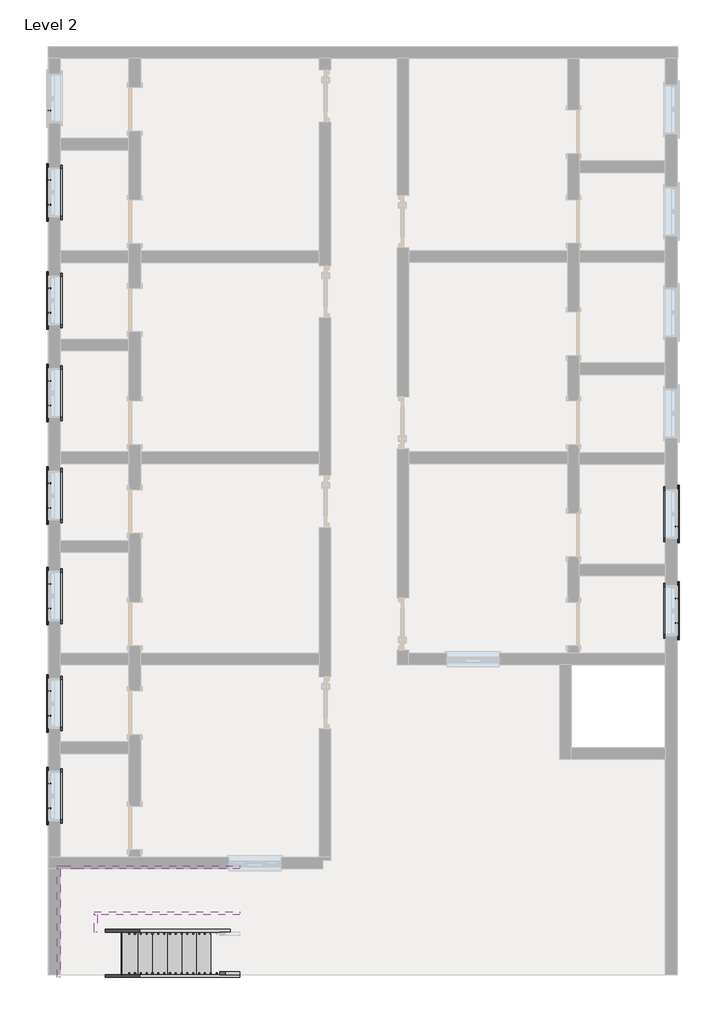
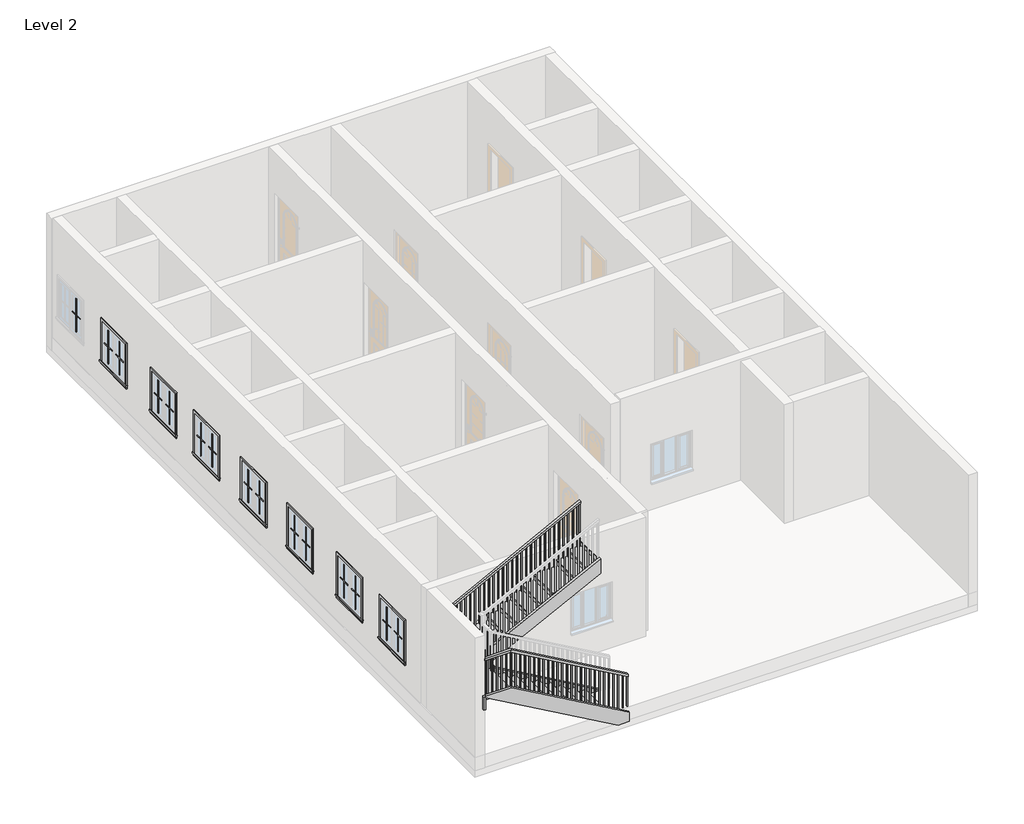
# One storey, part 3 of 4: 36 proxies, 6 members, 1 railing, 1 stair flight.
"""IFC4 building model written with IfcOpenShell, lengths in millimetres."""

from ifc_helpers import new_model, si_unit, frame, origin, place, context, project, spatial, polyline, outline, extrude, faceted_brep, transform, mapped, element, save
from components import muntin_pattern_2x2_muntin_pattern_2x2_b3fe6957, muntin_pattern_2x2_muntin_pattern_2x2_3e0ecaf2, trim_window_exterior_flat_with_sill_41619996, trim_window_interior_flat_picture_frame_51c85655, stair_flight_618316a1

model = new_model("IFC4")

# Units and contexts
model_context = context("Model", 3, world=origin())
ifc_project = project(units=[si_unit("LENGTHUNIT", "METRE", prefix="MILLI")], contexts=[model_context])

# Site, building, storey
site = spatial("IfcSite", under=ifc_project)
building = spatial("IfcBuilding", under=site)
storey = spatial("IfcBuildingStorey", under=building, Name="Level 2", Elevation=3048.0)

# Proxies
placement = place(None, origin())
muntin_pattern_2x2_muntin_pattern_2x2_shape = muntin_pattern_2x2_muntin_pattern_2x2_b3fe6957(model_context)
element("IfcBuildingElementProxy", 1, Name="Muntin Pattern_2x2 : Muntin Pattern_2x2", ObjectType="Muntin Pattern_2x2 : Muntin Pattern_2x2", at=placement, inside=storey, context=model_context, shape_type="MappedRepresentation", body=[
    mapped(muntin_pattern_2x2_muntin_pattern_2x2_shape, transform((-6438.8858866, 6882.8274728, 4032.25), x_axis=(0.0, 1.0, 0.0), y_axis=(-1.0, 0.0, 0.0), z_axis=(0.0, 0.0, 1.0))),
])
element("IfcBuildingElementProxy", 2, Name="Muntin Pattern_2x2 : Muntin Pattern_2x2", ObjectType="Muntin Pattern_2x2 : Muntin Pattern_2x2", at=placement, inside=storey, context=model_context, shape_type="MappedRepresentation", body=[
    mapped(muntin_pattern_2x2_muntin_pattern_2x2_shape, transform((-6438.8858866, 5244.5274728, 4032.25), x_axis=(0.0, 1.0, 0.0), y_axis=(-1.0, 0.0, 0.0), z_axis=(0.0, 0.0, 1.0))),
])
element("IfcBuildingElementProxy", 3, Name="Muntin Pattern_2x2 : Muntin Pattern_2x2", ObjectType="Muntin Pattern_2x2 : Muntin Pattern_2x2", at=placement, inside=storey, context=model_context, shape_type="MappedRepresentation", body=[
    mapped(muntin_pattern_2x2_muntin_pattern_2x2_shape, transform((-6438.8858866, 3360.4810874, 4032.25), x_axis=(0.0, 1.0, 0.0), y_axis=(-1.0, 0.0, 0.0), z_axis=(0.0, 0.0, 1.0))),
])
element("IfcBuildingElementProxy", 4, Name="Muntin Pattern_2x2 : Muntin Pattern_2x2", ObjectType="Muntin Pattern_2x2 : Muntin Pattern_2x2", at=placement, inside=storey, context=model_context, shape_type="MappedRepresentation", body=[
    mapped(muntin_pattern_2x2_muntin_pattern_2x2_shape, transform((-6438.8858866, 1745.426343, 4032.25), x_axis=(0.0, 1.0, 0.0), y_axis=(-1.0, 0.0, 0.0), z_axis=(0.0, 0.0, 1.0))),
])
element("IfcBuildingElementProxy", 5, Name="Muntin Pattern_2x2 : Muntin Pattern_2x2", ObjectType="Muntin Pattern_2x2 : Muntin Pattern_2x2", at=placement, inside=storey, context=model_context, shape_type="MappedRepresentation", body=[
    mapped(muntin_pattern_2x2_muntin_pattern_2x2_shape, transform((-6438.8858866, -38.6725272, 4032.25), x_axis=(0.0, 1.0, 0.0), y_axis=(-1.0, 0.0, 0.0), z_axis=(0.0, 0.0, 1.0))),
])
element("IfcBuildingElementProxy", 6, Name="Muntin Pattern_2x2 : Muntin Pattern_2x2", ObjectType="Muntin Pattern_2x2 : Muntin Pattern_2x2", at=placement, inside=storey, context=model_context, shape_type="MappedRepresentation", body=[
    mapped(muntin_pattern_2x2_muntin_pattern_2x2_shape, transform((-6438.8858866, -1791.2725272, 4032.25), x_axis=(0.0, 1.0, 0.0), y_axis=(-1.0, 0.0, 0.0), z_axis=(0.0, 0.0, 1.0))),
])
element("IfcBuildingElementProxy", 7, Name="Muntin Pattern_2x2 : Muntin Pattern_2x2", ObjectType="Muntin Pattern_2x2 : Muntin Pattern_2x2", at=placement, inside=storey, context=model_context, shape_type="MappedRepresentation", body=[
    mapped(muntin_pattern_2x2_muntin_pattern_2x2_shape, transform((-6438.8858866, -3658.1725272, 4032.25), x_axis=(0.0, 1.0, 0.0), y_axis=(-1.0, 0.0, 0.0), z_axis=(0.0, 0.0, 1.0))),
])
element("IfcBuildingElementProxy", 8, Name="Muntin Pattern_2x2 : Muntin Pattern_2x2", ObjectType="Muntin Pattern_2x2 : Muntin Pattern_2x2", at=placement, inside=storey, context=model_context, shape_type="MappedRepresentation", body=[
    mapped(muntin_pattern_2x2_muntin_pattern_2x2_shape, transform((-6438.8858866, -5271.0725272, 4032.25), x_axis=(0.0, 1.0, 0.0), y_axis=(-1.0, 0.0, 0.0), z_axis=(0.0, 0.0, 1.0))),
])
element("IfcBuildingElementProxy", 9, Name="Muntin Pattern_2x2 : Muntin Pattern_2x2", ObjectType="Muntin Pattern_2x2 : Muntin Pattern_2x2", at=placement, inside=storey, context=model_context, shape_type="MappedRepresentation", body=[
    mapped(muntin_pattern_2x2_muntin_pattern_2x2_shape, transform((4489.4641134, -1616.6475272, 4032.25), x_axis=(0.0, -1.0, 0.0), y_axis=(1.0, 0.0, 0.0), z_axis=(0.0, 0.0, 1.0))),
])
muntin_pattern_2x2_muntin_pattern_2x2_2_shape = muntin_pattern_2x2_muntin_pattern_2x2_3e0ecaf2(model_context)
element("IfcBuildingElementProxy", 10, Name="Muntin Pattern_2x2 : Muntin Pattern_2x2", ObjectType="Muntin Pattern_2x2 : Muntin Pattern_2x2", at=placement, inside=storey, context=model_context, shape_type="MappedRepresentation", body=[
    mapped(muntin_pattern_2x2_muntin_pattern_2x2_2_shape, transform((-6438.8858866, 5673.1524728, 4032.25), x_axis=(0.0, -1.0, 0.0), y_axis=(1.0, 0.0, 0.0), z_axis=(0.0, 0.0, 1.0))),
])
element("IfcBuildingElementProxy", 11, Name="Muntin Pattern_2x2 : Muntin Pattern_2x2", ObjectType="Muntin Pattern_2x2 : Muntin Pattern_2x2", at=placement, inside=storey, context=model_context, shape_type="MappedRepresentation", body=[
    mapped(muntin_pattern_2x2_muntin_pattern_2x2_2_shape, transform((-6438.8858866, 3789.1060874, 4032.25), x_axis=(0.0, -1.0, 0.0), y_axis=(1.0, 0.0, 0.0), z_axis=(0.0, 0.0, 1.0))),
])
element("IfcBuildingElementProxy", 12, Name="Muntin Pattern_2x2 : Muntin Pattern_2x2", ObjectType="Muntin Pattern_2x2 : Muntin Pattern_2x2", at=placement, inside=storey, context=model_context, shape_type="MappedRepresentation", body=[
    mapped(muntin_pattern_2x2_muntin_pattern_2x2_2_shape, transform((-6438.8858866, 2174.051343, 4032.25), x_axis=(0.0, -1.0, 0.0), y_axis=(1.0, 0.0, 0.0), z_axis=(0.0, 0.0, 1.0))),
])
element("IfcBuildingElementProxy", 13, Name="Muntin Pattern_2x2 : Muntin Pattern_2x2", ObjectType="Muntin Pattern_2x2 : Muntin Pattern_2x2", at=placement, inside=storey, context=model_context, shape_type="MappedRepresentation", body=[
    mapped(muntin_pattern_2x2_muntin_pattern_2x2_2_shape, transform((-6438.8858866, 389.9524728, 4032.25), x_axis=(0.0, -1.0, 0.0), y_axis=(1.0, 0.0, 0.0), z_axis=(0.0, 0.0, 1.0))),
])
element("IfcBuildingElementProxy", 14, Name="Muntin Pattern_2x2 : Muntin Pattern_2x2", ObjectType="Muntin Pattern_2x2 : Muntin Pattern_2x2", at=placement, inside=storey, context=model_context, shape_type="MappedRepresentation", body=[
    mapped(muntin_pattern_2x2_muntin_pattern_2x2_2_shape, transform((-6438.8858866, -1362.6475272, 4032.25), x_axis=(0.0, -1.0, 0.0), y_axis=(1.0, 0.0, 0.0), z_axis=(0.0, 0.0, 1.0))),
])
element("IfcBuildingElementProxy", 15, Name="Muntin Pattern_2x2 : Muntin Pattern_2x2", ObjectType="Muntin Pattern_2x2 : Muntin Pattern_2x2", at=placement, inside=storey, context=model_context, shape_type="MappedRepresentation", body=[
    mapped(muntin_pattern_2x2_muntin_pattern_2x2_2_shape, transform((-6438.8858866, -3229.5475272, 4032.25), x_axis=(0.0, -1.0, 0.0), y_axis=(1.0, 0.0, 0.0), z_axis=(0.0, 0.0, 1.0))),
])
element("IfcBuildingElementProxy", 16, Name="Muntin Pattern_2x2 : Muntin Pattern_2x2", ObjectType="Muntin Pattern_2x2 : Muntin Pattern_2x2", at=placement, inside=storey, context=model_context, shape_type="MappedRepresentation", body=[
    mapped(muntin_pattern_2x2_muntin_pattern_2x2_2_shape, transform((-6438.8858866, -4842.4475272, 4032.25), x_axis=(0.0, -1.0, 0.0), y_axis=(1.0, 0.0, 0.0), z_axis=(0.0, 0.0, 1.0))),
])
element("IfcBuildingElementProxy", 17, Name="Muntin Pattern_2x2 : Muntin Pattern_2x2", ObjectType="Muntin Pattern_2x2 : Muntin Pattern_2x2", at=placement, inside=storey, context=model_context, shape_type="MappedRepresentation", body=[
    mapped(muntin_pattern_2x2_muntin_pattern_2x2_2_shape, transform((4489.4641134, -2045.2725272, 4032.25), x_axis=(0.0, 1.0, 0.0), y_axis=(-1.0, 0.0, 0.0), z_axis=(0.0, 0.0, 1.0))),
])
element("IfcBuildingElementProxy", 18, Name="Muntin Pattern_2x2 : Muntin Pattern_2x2", ObjectType="Muntin Pattern_2x2 : Muntin Pattern_2x2", at=placement, inside=storey, context=model_context, shape_type="MappedRepresentation", body=[
    mapped(muntin_pattern_2x2_muntin_pattern_2x2_2_shape, transform((4489.4641134, -362.5225272, 4032.25), x_axis=(0.0, 1.0, 0.0), y_axis=(-1.0, 0.0, 0.0), z_axis=(0.0, 0.0, 1.0))),
])
trim_window_exterior_flat_with_sill_shape = trim_window_exterior_flat_with_sill_41619996(model_context)
element("IfcBuildingElementProxy", 19, Name="Trim-Window-Exterior-Flat : with Sill", ObjectType="Trim-Window-Exterior-Flat : with Sill", at=placement, inside=storey, context=model_context, shape_type="MappedRepresentation", body=[
    mapped(trim_window_exterior_flat_with_sill_shape, transform((-6448.4108866, 5458.8399728, 4876.8), x_axis=(0.0, -1.0, 0.0), y_axis=(0.0, 0.0, 1.0), z_axis=(-1.0, 0.0, 0.0))),
])
element("IfcBuildingElementProxy", 20, Name="Trim-Window-Exterior-Flat : with Sill", ObjectType="Trim-Window-Exterior-Flat : with Sill", at=placement, inside=storey, context=model_context, shape_type="MappedRepresentation", body=[
    mapped(trim_window_exterior_flat_with_sill_shape, transform((-6448.4108866, 3574.7935874, 4876.8), x_axis=(0.0, -1.0, 0.0), y_axis=(0.0, 0.0, 1.0), z_axis=(-1.0, 0.0, 0.0))),
])
element("IfcBuildingElementProxy", 21, Name="Trim-Window-Exterior-Flat : with Sill", ObjectType="Trim-Window-Exterior-Flat : with Sill", at=placement, inside=storey, context=model_context, shape_type="MappedRepresentation", body=[
    mapped(trim_window_exterior_flat_with_sill_shape, transform((-6448.4108866, 1959.738843, 4876.8), x_axis=(0.0, -1.0, 0.0), y_axis=(0.0, 0.0, 1.0), z_axis=(-1.0, 0.0, 0.0))),
])
element("IfcBuildingElementProxy", 22, Name="Trim-Window-Exterior-Flat : with Sill", ObjectType="Trim-Window-Exterior-Flat : with Sill", at=placement, inside=storey, context=model_context, shape_type="MappedRepresentation", body=[
    mapped(trim_window_exterior_flat_with_sill_shape, transform((-6448.4108866, 175.6399728, 4876.8), x_axis=(0.0, -1.0, 0.0), y_axis=(0.0, 0.0, 1.0), z_axis=(-1.0, 0.0, 0.0))),
])
element("IfcBuildingElementProxy", 23, Name="Trim-Window-Exterior-Flat : with Sill", ObjectType="Trim-Window-Exterior-Flat : with Sill", at=placement, inside=storey, context=model_context, shape_type="MappedRepresentation", body=[
    mapped(trim_window_exterior_flat_with_sill_shape, transform((-6448.4108866, -1576.9600272, 4876.8), x_axis=(0.0, -1.0, 0.0), y_axis=(0.0, 0.0, 1.0), z_axis=(-1.0, 0.0, 0.0))),
])
element("IfcBuildingElementProxy", 24, Name="Trim-Window-Exterior-Flat : with Sill", ObjectType="Trim-Window-Exterior-Flat : with Sill", at=placement, inside=storey, context=model_context, shape_type="MappedRepresentation", body=[
    mapped(trim_window_exterior_flat_with_sill_shape, transform((-6448.4108866, -3443.8600272, 4876.8), x_axis=(0.0, -1.0, 0.0), y_axis=(0.0, 0.0, 1.0), z_axis=(-1.0, 0.0, 0.0))),
])
element("IfcBuildingElementProxy", 25, Name="Trim-Window-Exterior-Flat : with Sill", ObjectType="Trim-Window-Exterior-Flat : with Sill", at=placement, inside=storey, context=model_context, shape_type="MappedRepresentation", body=[
    mapped(trim_window_exterior_flat_with_sill_shape, transform((-6448.4108866, -5056.7600272, 4876.8), x_axis=(0.0, -1.0, 0.0), y_axis=(0.0, 0.0, 1.0), z_axis=(-1.0, 0.0, 0.0))),
])
element("IfcBuildingElementProxy", 26, Name="Trim-Window-Exterior-Flat : with Sill", ObjectType="Trim-Window-Exterior-Flat : with Sill", at=placement, inside=storey, context=model_context, shape_type="MappedRepresentation", body=[
    mapped(trim_window_exterior_flat_with_sill_shape, transform((4498.9891134, -1830.9600272, 4876.8), x_axis=(0.0, 1.0, 0.0), y_axis=(0.0, 0.0, 1.0), z_axis=(1.0, 0.0, 0.0))),
])
element("IfcBuildingElementProxy", 27, Name="Trim-Window-Exterior-Flat : with Sill", ObjectType="Trim-Window-Exterior-Flat : with Sill", at=placement, inside=storey, context=model_context, shape_type="MappedRepresentation", body=[
    mapped(trim_window_exterior_flat_with_sill_shape, transform((4498.9891134, -148.2100272, 4876.8), x_axis=(0.0, 1.0, 0.0), y_axis=(0.0, 0.0, 1.0), z_axis=(1.0, 0.0, 0.0))),
])
trim_window_interior_flat_picture_frame_shape = trim_window_interior_flat_picture_frame_51c85655(model_context)
element("IfcBuildingElementProxy", 28, Name="Trim-Window-Interior-Flat : Picture Frame", ObjectType="Trim-Window-Interior-Flat : Picture Frame", at=placement, inside=storey, context=model_context, shape_type="MappedRepresentation", body=[
    mapped(trim_window_interior_flat_picture_frame_shape, transform((-6245.2108866, 5458.8399728, 4876.8), x_axis=(0.0, 1.0, 0.0), y_axis=(0.0, 0.0, 1.0), z_axis=(1.0, 0.0, 0.0))),
])
element("IfcBuildingElementProxy", 29, Name="Trim-Window-Interior-Flat : Picture Frame", ObjectType="Trim-Window-Interior-Flat : Picture Frame", at=placement, inside=storey, context=model_context, shape_type="MappedRepresentation", body=[
    mapped(trim_window_interior_flat_picture_frame_shape, transform((-6245.2108866, 3574.7935874, 4876.8), x_axis=(0.0, 1.0, 0.0), y_axis=(0.0, 0.0, 1.0), z_axis=(1.0, 0.0, 0.0))),
])
element("IfcBuildingElementProxy", 30, Name="Trim-Window-Interior-Flat : Picture Frame", ObjectType="Trim-Window-Interior-Flat : Picture Frame", at=placement, inside=storey, context=model_context, shape_type="MappedRepresentation", body=[
    mapped(trim_window_interior_flat_picture_frame_shape, transform((-6245.2108866, 1959.738843, 4876.8), x_axis=(0.0, 1.0, 0.0), y_axis=(0.0, 0.0, 1.0), z_axis=(1.0, 0.0, 0.0))),
])
element("IfcBuildingElementProxy", 31, Name="Trim-Window-Interior-Flat : Picture Frame", ObjectType="Trim-Window-Interior-Flat : Picture Frame", at=placement, inside=storey, context=model_context, shape_type="MappedRepresentation", body=[
    mapped(trim_window_interior_flat_picture_frame_shape, transform((-6245.2108866, 175.6399728, 4876.8), x_axis=(0.0, 1.0, 0.0), y_axis=(0.0, 0.0, 1.0), z_axis=(1.0, 0.0, 0.0))),
])
element("IfcBuildingElementProxy", 32, Name="Trim-Window-Interior-Flat : Picture Frame", ObjectType="Trim-Window-Interior-Flat : Picture Frame", at=placement, inside=storey, context=model_context, shape_type="MappedRepresentation", body=[
    mapped(trim_window_interior_flat_picture_frame_shape, transform((-6245.2108866, -1576.9600272, 4876.8), x_axis=(0.0, 1.0, 0.0), y_axis=(0.0, 0.0, 1.0), z_axis=(1.0, 0.0, 0.0))),
])
element("IfcBuildingElementProxy", 33, Name="Trim-Window-Interior-Flat : Picture Frame", ObjectType="Trim-Window-Interior-Flat : Picture Frame", at=placement, inside=storey, context=model_context, shape_type="MappedRepresentation", body=[
    mapped(trim_window_interior_flat_picture_frame_shape, transform((-6245.2108866, -3443.8600272, 4876.8), x_axis=(0.0, 1.0, 0.0), y_axis=(0.0, 0.0, 1.0), z_axis=(1.0, 0.0, 0.0))),
])
element("IfcBuildingElementProxy", 34, Name="Trim-Window-Interior-Flat : Picture Frame", ObjectType="Trim-Window-Interior-Flat : Picture Frame", at=placement, inside=storey, context=model_context, shape_type="MappedRepresentation", body=[
    mapped(trim_window_interior_flat_picture_frame_shape, transform((-6245.2108866, -5056.7600272, 4876.8), x_axis=(0.0, 1.0, 0.0), y_axis=(0.0, 0.0, 1.0), z_axis=(1.0, 0.0, 0.0))),
])
element("IfcBuildingElementProxy", 35, Name="Trim-Window-Interior-Flat : Picture Frame", ObjectType="Trim-Window-Interior-Flat : Picture Frame", at=placement, inside=storey, context=model_context, shape_type="MappedRepresentation", body=[
    mapped(trim_window_interior_flat_picture_frame_shape, transform((4295.7891134, -1830.9600272, 4876.8), x_axis=(0.0, -1.0, 0.0), y_axis=(0.0, 0.0, 1.0), z_axis=(-1.0, 0.0, 0.0))),
])
element("IfcBuildingElementProxy", 36, Name="Trim-Window-Interior-Flat : Picture Frame", ObjectType="Trim-Window-Interior-Flat : Picture Frame", at=placement, inside=storey, context=model_context, shape_type="MappedRepresentation", body=[
    mapped(trim_window_interior_flat_picture_frame_shape, transform((4295.7891134, -148.2100272, 4876.8), x_axis=(0.0, -1.0, 0.0), y_axis=(0.0, 0.0, 1.0), z_axis=(-1.0, 0.0, 0.0))),
])

# Members
element("IfcMember", 37, ObjectType="Stringer - 2\" Width", at=placement, inside=storey, context=model_context, shape_type="SweptSolid", body=[
    extrude(outline(polyline([(3048.0, -3117.2664982), (3256.974685, -3117.2664982), (4720.7714286, -5678.9107995), (4720.7714286, -6245.2108866), (4693.3177409, -6245.2108866), (3048.0, -3365.9048399), (3048.0, -3117.2664982)])), frame((0.0, -8219.0600272, 0.0), z_axis=(0.0, 1.0, 0.0), x_axis=(0.0, 0.0, 1.0)), (0.0, 0.0, 1.0), 50.8),
])
element("IfcMember", 38, ObjectType="Stringer - 2\" Width", at=placement, inside=storey, context=model_context, shape_type="SweptSolid", body=[
    extrude(outline(polyline([(-6245.2108866, -8219.0600272), (-6296.0108866, -8219.0600272), (-6296.0108866, -6326.7600272), (-6245.2108866, -6326.7600272), (-6245.2108866, -8219.0600272)])), frame((0.0, 0.0, 4415.9714286), z_axis=(0.0, 0.0, 1.0), x_axis=(1.0, 0.0, 0.0)), (0.0, 0.0, 1.0), 304.8),
])
element("IfcMember", 39, ObjectType="Stringer - 2\" Width", at=placement, inside=storey, context=model_context, shape_type="SweptSolid", body=[
    extrude(outline(polyline([(4523.8463219, -6296.0108866), (4415.9714286, -6296.0108866), (4415.9714286, -5835.3420022), (5796.5812084, -3117.2664982), (6138.4466461, -3117.2664982), (4523.8463219, -6296.0108866)])), frame((0.0, -6326.7600272, 0.0), z_axis=(0.0, 1.0, 0.0), x_axis=(0.0, 0.0, 1.0)), (0.0, 0.0, 1.0), 50.8),
])
element("IfcMember", 40, ObjectType="Stringer - 2\" Width", at=placement, inside=storey, context=model_context, shape_type="SweptSolid", body=[
    extrude(outline(polyline([(3048.0, -3117.2664982), (3256.974685, -3117.2664982), (4679.374685, -5606.4664982), (4328.3209476, -5606.4664982), (3048.0, -3365.9048399), (3048.0, -3117.2664982)])), frame((0.0, -7431.6600272, 0.0), z_axis=(0.0, 1.0, 0.0), x_axis=(0.0, 0.0, 1.0)), (0.0, 0.0, 1.0), 50.8),
])
element("IfcMember", 41, ObjectType="Stringer - 2\" Width", at=placement, inside=storey, context=model_context, shape_type="SweptSolid", body=[
    extrude(outline(polyline([(-5606.4664982, -7431.6600272), (-5657.2664982, -7431.6600272), (-5657.2664982, -7126.8600272), (-5606.4664982, -7126.8600272), (-5606.4664982, -7431.6600272)])), frame((0.0, 0.0, 4415.9714286), z_axis=(0.0, 0.0, 1.0), x_axis=(1.0, 0.0, 0.0)), (0.0, 0.0, 1.0), 304.8),
])
element("IfcMember", 42, ObjectType="Stringer - 2\" Width", at=placement, inside=storey, context=model_context, shape_type="SweptSolid", body=[
    extrude(outline(polyline([(4848.287916, -5657.2664982), (4506.4224783, -5657.2664982), (5796.5812084, -3117.2664982), (6138.4466461, -3117.2664982), (4848.287916, -5657.2664982)])), frame((0.0, -7126.8600272, 0.0), z_axis=(0.0, 1.0, 0.0), x_axis=(0.0, 0.0, 1.0)), (0.0, 0.0, 1.0), 50.8),
])

# Railing
element("IfcRailing", 43, ObjectType="Handrail - Rectangular", at=placement, inside=storey, context=model_context, shape_type="SolidModel", body=[
    faceted_brep([(-3117.2664982, -8168.2600272, 4107.5428571), (-3117.2664982, -8168.2600272, 4049.0339009), (-3117.2664982, -8117.4600272, 4049.0339009), (-3117.2664982, -8117.4600272, 4107.5428571), (-5657.2664982, -8168.2600272, 5558.9714286), (-5670.7571716, -8168.2600272, 5508.1714286), (-5670.7571716, -8117.4600272, 5508.1714286), (-5657.2664982, -8117.4600272, 5558.9714286), (-6245.2108866, -8168.2600272, 5558.9714286), (-6245.2108866, -8168.2600272, 5508.1714286), (-6194.4108866, -8117.4600272, 5508.1714286), (-6194.4108866, -8117.4600272, 5558.9714286), (-6245.2108866, -6326.7600272, 5558.9714286), (-6245.2108866, -6326.7600272, 5508.1714286), (-6194.4108866, -6377.5600272, 5508.1714286), (-6194.4108866, -6377.5600272, 5558.9714286), (-5939.4887204, -6326.7600272, 5558.9714286), (-5927.1913462, -6326.7600272, 5508.1714286), (-5927.1913462, -6377.5600272, 5508.1714286), (-5939.4887204, -6377.5600272, 5558.9714286), (-3117.2664982, -6326.7600272, 7010.4), (-3117.2664982, -6377.5600272, 7010.4), (-3117.2664982, -6377.5600272, 6953.2756361), (-3117.2664982, -6326.7600272, 6953.2756361)], [[[0, 1, 2, 3]], [[1, 0, 4, 5]], [[2, 1, 5, 6]], [[3, 2, 6, 7]], [[0, 3, 7, 4]], [[5, 4, 8, 9]], [[6, 5, 9, 10]], [[7, 6, 10, 11]], [[4, 7, 11, 8]], [[9, 8, 12, 13]], [[10, 9, 13, 14]], [[11, 10, 14, 15]], [[8, 11, 15, 12]], [[13, 12, 16, 17]], [[14, 13, 17, 18]], [[15, 14, 18, 19]], [[12, 15, 19, 16]], [[20, 21, 22, 23]], [[17, 16, 20, 23]], [[18, 17, 23, 22]], [[19, 18, 22, 21]], [[16, 19, 21, 20]]]),
    extrude(outline(polyline([(6920.325665, -3181.3358866), (5950.8571429, -3181.3358866), (5950.8571429, -3162.2858866), (6930.1228078, -3162.2858866), (6920.325665, -3181.3358866)])), frame((0.0, -6361.6850272, 0.0), z_axis=(0.0, 1.0, 0.0), x_axis=(0.0, 0.0, 1.0)), (0.0, 0.0, 1.0), 19.05),
    extrude(outline(polyline([(6868.0742364, -3282.9358866), (5950.8571429, -3282.9358866), (5950.8571429, -3263.8858866), (6877.8713793, -3263.8858866), (6868.0742364, -3282.9358866)])), frame((0.0, -6361.6850272, 0.0), z_axis=(0.0, 1.0, 0.0), x_axis=(0.0, 0.0, 1.0)), (0.0, 0.0, 1.0), 19.05),
    extrude(outline(polyline([(6815.8228078, -3384.5358866), (5805.7142857, -3384.5358866), (5805.7142857, -3365.4858866), (6825.6199507, -3365.4858866), (6815.8228078, -3384.5358866)])), frame((0.0, -6361.6850272, 0.0), z_axis=(0.0, 1.0, 0.0), x_axis=(0.0, 0.0, 1.0)), (0.0, 0.0, 1.0), 19.05),
    extrude(outline(polyline([(6763.5713793, -3486.1358866), (5805.7142857, -3486.1358866), (5805.7142857, -3467.0858866), (6773.3685221, -3467.0858866), (6763.5713793, -3486.1358866)])), frame((0.0, -6361.6850272, 0.0), z_axis=(0.0, 1.0, 0.0), x_axis=(0.0, 0.0, 1.0)), (0.0, 0.0, 1.0), 19.05),
    extrude(outline(polyline([(6711.3199507, -3587.7358866), (5805.7142857, -3587.7358866), (5805.7142857, -3568.6858866), (6721.1170935, -3568.6858866), (6711.3199507, -3587.7358866)])), frame((0.0, -6361.6850272, 0.0), z_axis=(0.0, 1.0, 0.0), x_axis=(0.0, 0.0, 1.0)), (0.0, 0.0, 1.0), 19.05),
    extrude(outline(polyline([(6659.0685221, -3689.3358866), (5660.5714286, -3689.3358866), (5660.5714286, -3670.2858866), (6668.865665, -3670.2858866), (6659.0685221, -3689.3358866)])), frame((0.0, -6361.6850272, 0.0), z_axis=(0.0, 1.0, 0.0), x_axis=(0.0, 0.0, 1.0)), (0.0, 0.0, 1.0), 19.05),
    extrude(outline(polyline([(6606.8170935, -3790.9358866), (5660.5714286, -3790.9358866), (5660.5714286, -3771.8858866), (6616.6142364, -3771.8858866), (6606.8170935, -3790.9358866)])), frame((0.0, -6361.6850272, 0.0), z_axis=(0.0, 1.0, 0.0), x_axis=(0.0, 0.0, 1.0)), (0.0, 0.0, 1.0), 19.05),
    extrude(outline(polyline([(6554.565665, -3892.5358866), (5660.5714286, -3892.5358866), (5660.5714286, -3873.4858866), (6564.3628078, -3873.4858866), (6554.565665, -3892.5358866)])), frame((0.0, -6361.6850272, 0.0), z_axis=(0.0, 1.0, 0.0), x_axis=(0.0, 0.0, 1.0)), (0.0, 0.0, 1.0), 19.05),
    extrude(outline(polyline([(6502.3142364, -3994.1358866), (5660.5714286, -3994.1358866), (5660.5714286, -3975.0858866), (6512.1113793, -3975.0858866), (6502.3142364, -3994.1358866)])), frame((0.0, -6361.6850272, 0.0), z_axis=(0.0, 1.0, 0.0), x_axis=(0.0, 0.0, 1.0)), (0.0, 0.0, 1.0), 19.05),
    extrude(outline(polyline([(6450.0628078, -4095.7358866), (5660.5714286, -4095.7358866), (5660.5714286, -4076.6858866), (6459.8599507, -4076.6858866), (6450.0628078, -4095.7358866)])), frame((0.0, -6361.6850272, 0.0), z_axis=(0.0, 1.0, 0.0), x_axis=(0.0, 0.0, 1.0)), (0.0, 0.0, 1.0), 19.05),
    extrude(outline(polyline([(6397.8113793, -4197.3358866), (5515.4285714, -4197.3358866), (5515.4285714, -4178.2858866), (6407.6085221, -4178.2858866), (6397.8113793, -4197.3358866)])), frame((0.0, -6361.6850272, 0.0), z_axis=(0.0, 1.0, 0.0), x_axis=(0.0, 0.0, 1.0)), (0.0, 0.0, 1.0), 19.05),
    extrude(outline(polyline([(6345.5599507, -4298.9358866), (5515.4285714, -4298.9358866), (5515.4285714, -4279.8858866), (6355.3570935, -4279.8858866), (6345.5599507, -4298.9358866)])), frame((0.0, -6361.6850272, 0.0), z_axis=(0.0, 1.0, 0.0), x_axis=(0.0, 0.0, 1.0)), (0.0, 0.0, 1.0), 19.05),
    extrude(outline(polyline([(6293.3085221, -4400.5358866), (5370.2857143, -4400.5358866), (5370.2857143, -4381.4858866), (6303.105665, -4381.4858866), (6293.3085221, -4400.5358866)])), frame((0.0, -6361.6850272, 0.0), z_axis=(0.0, 1.0, 0.0), x_axis=(0.0, 0.0, 1.0)), (0.0, 0.0, 1.0), 19.05),
    extrude(outline(polyline([(6241.0570935, -4502.1358866), (5370.2857143, -4502.1358866), (5370.2857143, -4483.0858866), (6250.8542364, -4483.0858866), (6241.0570935, -4502.1358866)])), frame((0.0, -6361.6850272, 0.0), z_axis=(0.0, 1.0, 0.0), x_axis=(0.0, 0.0, 1.0)), (0.0, 0.0, 1.0), 19.05),
    extrude(outline(polyline([(6188.805665, -4603.7358866), (5370.2857143, -4603.7358866), (5370.2857143, -4584.6858866), (6198.6028078, -4584.6858866), (6188.805665, -4603.7358866)])), frame((0.0, -6361.6850272, 0.0), z_axis=(0.0, 1.0, 0.0), x_axis=(0.0, 0.0, 1.0)), (0.0, 0.0, 1.0), 19.05),
    extrude(outline(polyline([(6136.5542364, -4705.3358866), (5225.1428571, -4705.3358866), (5225.1428571, -4686.2858866), (6146.3513793, -4686.2858866), (6136.5542364, -4705.3358866)])), frame((0.0, -6361.6850272, 0.0), z_axis=(0.0, 1.0, 0.0), x_axis=(0.0, 0.0, 1.0)), (0.0, 0.0, 1.0), 19.05),
    extrude(outline(polyline([(6084.3028078, -4806.9358866), (5225.1428571, -4806.9358866), (5225.1428571, -4787.8858866), (6094.0999507, -4787.8858866), (6084.3028078, -4806.9358866)])), frame((0.0, -6361.6850272, 0.0), z_axis=(0.0, 1.0, 0.0), x_axis=(0.0, 0.0, 1.0)), (0.0, 0.0, 1.0), 19.05),
    extrude(outline(polyline([(6032.0513793, -4908.5358866), (5080.0, -4908.5358866), (5080.0, -4889.4858866), (6041.8485221, -4889.4858866), (6032.0513793, -4908.5358866)])), frame((0.0, -6361.6850272, 0.0), z_axis=(0.0, 1.0, 0.0), x_axis=(0.0, 0.0, 1.0)), (0.0, 0.0, 1.0), 19.05),
    extrude(outline(polyline([(5979.7999507, -5010.1358866), (5080.0, -5010.1358866), (5080.0, -4991.0858866), (5989.5970935, -4991.0858866), (5979.7999507, -5010.1358866)])), frame((0.0, -6361.6850272, 0.0), z_axis=(0.0, 1.0, 0.0), x_axis=(0.0, 0.0, 1.0)), (0.0, 0.0, 1.0), 19.05),
    extrude(outline(polyline([(5927.5485221, -5111.7358866), (5080.0, -5111.7358866), (5080.0, -5092.6858866), (5937.345665, -5092.6858866), (5927.5485221, -5111.7358866)])), frame((0.0, -6361.6850272, 0.0), z_axis=(0.0, 1.0, 0.0), x_axis=(0.0, 0.0, 1.0)), (0.0, 0.0, 1.0), 19.05),
    extrude(outline(polyline([(5875.2970935, -5213.3358866), (4934.8571429, -5213.3358866), (4934.8571429, -5194.2858866), (5885.0942364, -5194.2858866), (5875.2970935, -5213.3358866)])), frame((0.0, -6361.6850272, 0.0), z_axis=(0.0, 1.0, 0.0), x_axis=(0.0, 0.0, 1.0)), (0.0, 0.0, 1.0), 19.05),
    extrude(outline(polyline([(5823.045665, -5314.9358866), (4934.8571429, -5314.9358866), (4934.8571429, -5295.8858866), (5832.8428078, -5295.8858866), (5823.045665, -5314.9358866)])), frame((0.0, -6361.6850272, 0.0), z_axis=(0.0, 1.0, 0.0), x_axis=(0.0, 0.0, 1.0)), (0.0, 0.0, 1.0), 19.05),
    extrude(outline(polyline([(5770.7942364, -5416.5358866), (4789.7142857, -5416.5358866), (4789.7142857, -5397.4858866), (5780.5913793, -5397.4858866), (5770.7942364, -5416.5358866)])), frame((0.0, -6361.6850272, 0.0), z_axis=(0.0, 1.0, 0.0), x_axis=(0.0, 0.0, 1.0)), (0.0, 0.0, 1.0), 19.05),
    extrude(outline(polyline([(5718.5428078, -5518.1358866), (4789.7142857, -5518.1358866), (4789.7142857, -5499.0858866), (5728.3399507, -5499.0858866), (5718.5428078, -5518.1358866)])), frame((0.0, -6361.6850272, 0.0), z_axis=(0.0, 1.0, 0.0), x_axis=(0.0, 0.0, 1.0)), (0.0, 0.0, 1.0), 19.05),
    extrude(outline(polyline([(5666.2913793, -5619.7358866), (4789.7142857, -5619.7358866), (4789.7142857, -5600.6858866), (5676.0885221, -5600.6858866), (5666.2913793, -5619.7358866)])), frame((0.0, -6361.6850272, 0.0), z_axis=(0.0, 1.0, 0.0), x_axis=(0.0, 0.0, 1.0)), (0.0, 0.0, 1.0), 19.05),
    extrude(outline(polyline([(5614.0399507, -5721.3358866), (4644.5714286, -5721.3358866), (4644.5714286, -5702.2858866), (5623.8370935, -5702.2858866), (5614.0399507, -5721.3358866)])), frame((0.0, -6361.6850272, 0.0), z_axis=(0.0, 1.0, 0.0), x_axis=(0.0, 0.0, 1.0)), (0.0, 0.0, 1.0), 19.05),
    extrude(outline(polyline([(5561.7885221, -5822.9358866), (4644.5714286, -5822.9358866), (4644.5714286, -5803.8858866), (5571.585665, -5803.8858866), (5561.7885221, -5822.9358866)])), frame((0.0, -6361.6850272, 0.0), z_axis=(0.0, 1.0, 0.0), x_axis=(0.0, 0.0, 1.0)), (0.0, 0.0, 1.0), 19.05),
    extrude(outline(polyline([(5509.5370935, -5924.5358866), (4644.5714286, -5924.5358866), (4644.5714286, -5905.4858866), (5519.3342364, -5905.4858866), (5509.5370935, -5924.5358866)])), frame((0.0, -6361.6850272, 0.0), z_axis=(0.0, 1.0, 0.0), x_axis=(0.0, 0.0, 1.0)), (0.0, 0.0, 1.0), 19.05),
    extrude(outline(polyline([(-6026.1358866, -6342.6350272), (-6007.0858866, -6342.6350272), (-6007.0858866, -6361.6850272), (-6026.1358866, -6361.6850272), (-6026.1358866, -6342.6350272)])), frame((0.0, 0.0, 4644.5714286), z_axis=(0.0, 0.0, 1.0), x_axis=(1.0, 0.0, 0.0)), (0.0, 0.0, 1.0), 863.6),
    extrude(outline(polyline([(-6127.7358866, -6342.6350272), (-6108.6858866, -6342.6350272), (-6108.6858866, -6361.6850272), (-6127.7358866, -6361.6850272), (-6127.7358866, -6342.6350272)])), frame((0.0, 0.0, 4644.5714286), z_axis=(0.0, 0.0, 1.0), x_axis=(1.0, 0.0, 0.0)), (0.0, 0.0, 1.0), 863.6),
    extrude(outline(polyline([(-6229.3358866, -6425.1850272), (-6229.3358866, -6406.1350272), (-6210.2858866, -6406.1350272), (-6210.2858866, -6425.1850272), (-6229.3358866, -6425.1850272)])), frame((0.0, 0.0, 4644.5714286), z_axis=(0.0, 0.0, 1.0), x_axis=(1.0, 0.0, 0.0)), (0.0, 0.0, 1.0), 863.6),
    extrude(outline(polyline([(-6229.3358866, -6526.7850272), (-6229.3358866, -6507.7350272), (-6210.2858866, -6507.7350272), (-6210.2858866, -6526.7850272), (-6229.3358866, -6526.7850272)])), frame((0.0, 0.0, 4644.5714286), z_axis=(0.0, 0.0, 1.0), x_axis=(1.0, 0.0, 0.0)), (0.0, 0.0, 1.0), 863.6),
    extrude(outline(polyline([(-6229.3358866, -6628.3850272), (-6229.3358866, -6609.3350272), (-6210.2858866, -6609.3350272), (-6210.2858866, -6628.3850272), (-6229.3358866, -6628.3850272)])), frame((0.0, 0.0, 4644.5714286), z_axis=(0.0, 0.0, 1.0), x_axis=(1.0, 0.0, 0.0)), (0.0, 0.0, 1.0), 863.6),
    extrude(outline(polyline([(-6229.3358866, -6729.9850272), (-6229.3358866, -6710.9350272), (-6210.2858866, -6710.9350272), (-6210.2858866, -6729.9850272), (-6229.3358866, -6729.9850272)])), frame((0.0, 0.0, 4644.5714286), z_axis=(0.0, 0.0, 1.0), x_axis=(1.0, 0.0, 0.0)), (0.0, 0.0, 1.0), 863.6),
    extrude(outline(polyline([(-6229.3358866, -6831.5850272), (-6229.3358866, -6812.5350272), (-6210.2858866, -6812.5350272), (-6210.2858866, -6831.5850272), (-6229.3358866, -6831.5850272)])), frame((0.0, 0.0, 4644.5714286), z_axis=(0.0, 0.0, 1.0), x_axis=(1.0, 0.0, 0.0)), (0.0, 0.0, 1.0), 863.6),
    extrude(outline(polyline([(-6229.3358866, -6933.1850272), (-6229.3358866, -6914.1350272), (-6210.2858866, -6914.1350272), (-6210.2858866, -6933.1850272), (-6229.3358866, -6933.1850272)])), frame((0.0, 0.0, 4644.5714286), z_axis=(0.0, 0.0, 1.0), x_axis=(1.0, 0.0, 0.0)), (0.0, 0.0, 1.0), 863.6),
    extrude(outline(polyline([(-6229.3358866, -7034.7850272), (-6229.3358866, -7015.7350272), (-6210.2858866, -7015.7350272), (-6210.2858866, -7034.7850272), (-6229.3358866, -7034.7850272)])), frame((0.0, 0.0, 4644.5714286), z_axis=(0.0, 0.0, 1.0), x_axis=(1.0, 0.0, 0.0)), (0.0, 0.0, 1.0), 863.6),
    extrude(outline(polyline([(-6229.3358866, -7136.3850272), (-6229.3358866, -7117.3350272), (-6210.2858866, -7117.3350272), (-6210.2858866, -7136.3850272), (-6229.3358866, -7136.3850272)])), frame((0.0, 0.0, 4644.5714286), z_axis=(0.0, 0.0, 1.0), x_axis=(1.0, 0.0, 0.0)), (0.0, 0.0, 1.0), 863.6),
    extrude(outline(polyline([(-6229.3358866, -7237.9850272), (-6229.3358866, -7218.9350272), (-6210.2858866, -7218.9350272), (-6210.2858866, -7237.9850272), (-6229.3358866, -7237.9850272)])), frame((0.0, 0.0, 4644.5714286), z_axis=(0.0, 0.0, 1.0), x_axis=(1.0, 0.0, 0.0)), (0.0, 0.0, 1.0), 863.6),
    extrude(outline(polyline([(-6229.3358866, -7339.5850272), (-6229.3358866, -7320.5350272), (-6210.2858866, -7320.5350272), (-6210.2858866, -7339.5850272), (-6229.3358866, -7339.5850272)])), frame((0.0, 0.0, 4644.5714286), z_axis=(0.0, 0.0, 1.0), x_axis=(1.0, 0.0, 0.0)), (0.0, 0.0, 1.0), 863.6),
    extrude(outline(polyline([(-6229.3358866, -7441.1850272), (-6229.3358866, -7422.1350272), (-6210.2858866, -7422.1350272), (-6210.2858866, -7441.1850272), (-6229.3358866, -7441.1850272)])), frame((0.0, 0.0, 4644.5714286), z_axis=(0.0, 0.0, 1.0), x_axis=(1.0, 0.0, 0.0)), (0.0, 0.0, 1.0), 863.6),
    extrude(outline(polyline([(-6229.3358866, -7542.7850272), (-6229.3358866, -7523.7350272), (-6210.2858866, -7523.7350272), (-6210.2858866, -7542.7850272), (-6229.3358866, -7542.7850272)])), frame((0.0, 0.0, 4644.5714286), z_axis=(0.0, 0.0, 1.0), x_axis=(1.0, 0.0, 0.0)), (0.0, 0.0, 1.0), 863.6),
    extrude(outline(polyline([(-6229.3358866, -7644.3850272), (-6229.3358866, -7625.3350272), (-6210.2858866, -7625.3350272), (-6210.2858866, -7644.3850272), (-6229.3358866, -7644.3850272)])), frame((0.0, 0.0, 4644.5714286), z_axis=(0.0, 0.0, 1.0), x_axis=(1.0, 0.0, 0.0)), (0.0, 0.0, 1.0), 863.6),
    extrude(outline(polyline([(-6229.3358866, -7745.9850272), (-6229.3358866, -7726.9350272), (-6210.2858866, -7726.9350272), (-6210.2858866, -7745.9850272), (-6229.3358866, -7745.9850272)])), frame((0.0, 0.0, 4644.5714286), z_axis=(0.0, 0.0, 1.0), x_axis=(1.0, 0.0, 0.0)), (0.0, 0.0, 1.0), 863.6),
    extrude(outline(polyline([(-6229.3358866, -7847.5850272), (-6229.3358866, -7828.5350272), (-6210.2858866, -7828.5350272), (-6210.2858866, -7847.5850272), (-6229.3358866, -7847.5850272)])), frame((0.0, 0.0, 4644.5714286), z_axis=(0.0, 0.0, 1.0), x_axis=(1.0, 0.0, 0.0)), (0.0, 0.0, 1.0), 863.6),
    extrude(outline(polyline([(-6229.3358866, -7949.1850272), (-6229.3358866, -7930.1350272), (-6210.2858866, -7930.1350272), (-6210.2858866, -7949.1850272), (-6229.3358866, -7949.1850272)])), frame((0.0, 0.0, 4644.5714286), z_axis=(0.0, 0.0, 1.0), x_axis=(1.0, 0.0, 0.0)), (0.0, 0.0, 1.0), 863.6),
    extrude(outline(polyline([(-6229.3358866, -8050.7850272), (-6229.3358866, -8031.7350272), (-6210.2858866, -8031.7350272), (-6210.2858866, -8050.7850272), (-6229.3358866, -8050.7850272)])), frame((0.0, 0.0, 4644.5714286), z_axis=(0.0, 0.0, 1.0), x_axis=(1.0, 0.0, 0.0)), (0.0, 0.0, 1.0), 863.6),
    extrude(outline(polyline([(-6155.7414982, -8152.3850272), (-6174.7914982, -8152.3850272), (-6174.7914982, -8133.3350272), (-6155.7414982, -8133.3350272), (-6155.7414982, -8152.3850272)])), frame((0.0, 0.0, 4644.5714286), z_axis=(0.0, 0.0, 1.0), x_axis=(1.0, 0.0, 0.0)), (0.0, 0.0, 1.0), 863.6),
    extrude(outline(polyline([(-6054.1414982, -8152.3850272), (-6073.1914982, -8152.3850272), (-6073.1914982, -8133.3350272), (-6054.1414982, -8133.3350272), (-6054.1414982, -8152.3850272)])), frame((0.0, 0.0, 4644.5714286), z_axis=(0.0, 0.0, 1.0), x_axis=(1.0, 0.0, 0.0)), (0.0, 0.0, 1.0), 863.6),
    extrude(outline(polyline([(-5952.5414982, -8152.3850272), (-5971.5914982, -8152.3850272), (-5971.5914982, -8133.3350272), (-5952.5414982, -8133.3350272), (-5952.5414982, -8152.3850272)])), frame((0.0, 0.0, 4644.5714286), z_axis=(0.0, 0.0, 1.0), x_axis=(1.0, 0.0, 0.0)), (0.0, 0.0, 1.0), 863.6),
    extrude(outline(polyline([(-5850.9414982, -8152.3850272), (-5869.9914982, -8152.3850272), (-5869.9914982, -8133.3350272), (-5850.9414982, -8133.3350272), (-5850.9414982, -8152.3850272)])), frame((0.0, 0.0, 4644.5714286), z_axis=(0.0, 0.0, 1.0), x_axis=(1.0, 0.0, 0.0)), (0.0, 0.0, 1.0), 863.6),
    extrude(outline(polyline([(-5749.3414982, -8152.3850272), (-5768.3914982, -8152.3850272), (-5768.3914982, -8133.3350272), (-5749.3414982, -8133.3350272), (-5749.3414982, -8152.3850272)])), frame((0.0, 0.0, 4644.5714286), z_axis=(0.0, 0.0, 1.0), x_axis=(1.0, 0.0, 0.0)), (0.0, 0.0, 1.0), 863.6),
    extrude(outline(polyline([(5505.9053295, -5666.7914982), (4644.5714286, -5666.7914982), (4644.5714286, -5647.7414982), (5495.0196152, -5647.7414982), (5505.9053295, -5666.7914982)])), frame((0.0, -8152.3850272, 0.0), z_axis=(0.0, 1.0, 0.0), x_axis=(0.0, 0.0, 1.0)), (0.0, 0.0, 1.0), 19.05),
    extrude(outline(polyline([(5447.8481866, -5565.1914982), (4499.4285714, -5565.1914982), (4499.4285714, -5546.1414982), (5436.9624723, -5546.1414982), (5447.8481866, -5565.1914982)])), frame((0.0, -8152.3850272, 0.0), z_axis=(0.0, 1.0, 0.0), x_axis=(0.0, 0.0, 1.0)), (0.0, 0.0, 1.0), 19.05),
    extrude(outline(polyline([(5389.7910438, -5463.5914982), (4499.4285714, -5463.5914982), (4499.4285714, -5444.5414982), (5378.9053295, -5444.5414982), (5389.7910438, -5463.5914982)])), frame((0.0, -8152.3850272, 0.0), z_axis=(0.0, 1.0, 0.0), x_axis=(0.0, 0.0, 1.0)), (0.0, 0.0, 1.0), 19.05),
    extrude(outline(polyline([(5331.7339009, -5361.9914982), (4354.2857143, -5361.9914982), (4354.2857143, -5342.9414982), (5320.8481866, -5342.9414982), (5331.7339009, -5361.9914982)])), frame((0.0, -8152.3850272, 0.0), z_axis=(0.0, 1.0, 0.0), x_axis=(0.0, 0.0, 1.0)), (0.0, 0.0, 1.0), 19.05),
    extrude(outline(polyline([(5273.6767581, -5260.3914982), (4354.2857143, -5260.3914982), (4354.2857143, -5241.3414982), (5262.7910438, -5241.3414982), (5273.6767581, -5260.3914982)])), frame((0.0, -8152.3850272, 0.0), z_axis=(0.0, 1.0, 0.0), x_axis=(0.0, 0.0, 1.0)), (0.0, 0.0, 1.0), 19.05),
    extrude(outline(polyline([(5215.6196152, -5158.7914982), (4354.2857143, -5158.7914982), (4354.2857143, -5139.7414982), (5204.7339009, -5139.7414982), (5215.6196152, -5158.7914982)])), frame((0.0, -8152.3850272, 0.0), z_axis=(0.0, 1.0, 0.0), x_axis=(0.0, 0.0, 1.0)), (0.0, 0.0, 1.0), 19.05),
    extrude(outline(polyline([(5157.5624723, -5057.1914982), (4209.1428571, -5057.1914982), (4209.1428571, -5038.1414982), (5146.6767581, -5038.1414982), (5157.5624723, -5057.1914982)])), frame((0.0, -8152.3850272, 0.0), z_axis=(0.0, 1.0, 0.0), x_axis=(0.0, 0.0, 1.0)), (0.0, 0.0, 1.0), 19.05),
    extrude(outline(polyline([(5099.5053295, -4955.5914982), (4209.1428571, -4955.5914982), (4209.1428571, -4936.5414982), (5088.6196152, -4936.5414982), (5099.5053295, -4955.5914982)])), frame((0.0, -8152.3850272, 0.0), z_axis=(0.0, 1.0, 0.0), x_axis=(0.0, 0.0, 1.0)), (0.0, 0.0, 1.0), 19.05),
    extrude(outline(polyline([(5041.4481866, -4853.9914982), (4064.0, -4853.9914982), (4064.0, -4834.9414982), (5030.5624723, -4834.9414982), (5041.4481866, -4853.9914982)])), frame((0.0, -8152.3850272, 0.0), z_axis=(0.0, 1.0, 0.0), x_axis=(0.0, 0.0, 1.0)), (0.0, 0.0, 1.0), 19.05),
    extrude(outline(polyline([(4983.3910438, -4752.3914982), (4064.0, -4752.3914982), (4064.0, -4733.3414982), (4972.5053295, -4733.3414982), (4983.3910438, -4752.3914982)])), frame((0.0, -8152.3850272, 0.0), z_axis=(0.0, 1.0, 0.0), x_axis=(0.0, 0.0, 1.0)), (0.0, 0.0, 1.0), 19.05),
    extrude(outline(polyline([(4925.3339009, -4650.7914982), (4064.0, -4650.7914982), (4064.0, -4631.7414982), (4914.4481866, -4631.7414982), (4925.3339009, -4650.7914982)])), frame((0.0, -8152.3850272, 0.0), z_axis=(0.0, 1.0, 0.0), x_axis=(0.0, 0.0, 1.0)), (0.0, 0.0, 1.0), 19.05),
    extrude(outline(polyline([(4867.2767581, -4549.1914982), (3918.8571429, -4549.1914982), (3918.8571429, -4530.1414982), (4856.3910438, -4530.1414982), (4867.2767581, -4549.1914982)])), frame((0.0, -8152.3850272, 0.0), z_axis=(0.0, 1.0, 0.0), x_axis=(0.0, 0.0, 1.0)), (0.0, 0.0, 1.0), 19.05),
    extrude(outline(polyline([(4809.2196152, -4447.5914982), (3918.8571429, -4447.5914982), (3918.8571429, -4428.5414982), (4798.3339009, -4428.5414982), (4809.2196152, -4447.5914982)])), frame((0.0, -8152.3850272, 0.0), z_axis=(0.0, 1.0, 0.0), x_axis=(0.0, 0.0, 1.0)), (0.0, 0.0, 1.0), 19.05),
    extrude(outline(polyline([(4751.1624723, -4345.9914982), (3773.7142857, -4345.9914982), (3773.7142857, -4326.9414982), (4740.2767581, -4326.9414982), (4751.1624723, -4345.9914982)])), frame((0.0, -8152.3850272, 0.0), z_axis=(0.0, 1.0, 0.0), x_axis=(0.0, 0.0, 1.0)), (0.0, 0.0, 1.0), 19.05),
    extrude(outline(polyline([(4693.1053295, -4244.3914982), (3773.7142857, -4244.3914982), (3773.7142857, -4225.3414982), (4682.2196152, -4225.3414982), (4693.1053295, -4244.3914982)])), frame((0.0, -8152.3850272, 0.0), z_axis=(0.0, 1.0, 0.0), x_axis=(0.0, 0.0, 1.0)), (0.0, 0.0, 1.0), 19.05),
    extrude(outline(polyline([(4635.0481866, -4142.7914982), (3773.7142857, -4142.7914982), (3773.7142857, -4123.7414982), (4624.1624723, -4123.7414982), (4635.0481866, -4142.7914982)])), frame((0.0, -8152.3850272, 0.0), z_axis=(0.0, 1.0, 0.0), x_axis=(0.0, 0.0, 1.0)), (0.0, 0.0, 1.0), 19.05),
    extrude(outline(polyline([(4576.9910438, -4041.1914982), (3628.5714286, -4041.1914982), (3628.5714286, -4022.1414982), (4566.1053295, -4022.1414982), (4576.9910438, -4041.1914982)])), frame((0.0, -8152.3850272, 0.0), z_axis=(0.0, 1.0, 0.0), x_axis=(0.0, 0.0, 1.0)), (0.0, 0.0, 1.0), 19.05),
    extrude(outline(polyline([(4518.9339009, -3939.5914982), (3628.5714286, -3939.5914982), (3628.5714286, -3920.5414982), (4508.0481866, -3920.5414982), (4518.9339009, -3939.5914982)])), frame((0.0, -8152.3850272, 0.0), z_axis=(0.0, 1.0, 0.0), x_axis=(0.0, 0.0, 1.0)), (0.0, 0.0, 1.0), 19.05),
    extrude(outline(polyline([(4460.8767581, -3837.9914982), (3483.4285714, -3837.9914982), (3483.4285714, -3818.9414982), (4449.9910438, -3818.9414982), (4460.8767581, -3837.9914982)])), frame((0.0, -8152.3850272, 0.0), z_axis=(0.0, 1.0, 0.0), x_axis=(0.0, 0.0, 1.0)), (0.0, 0.0, 1.0), 19.05),
    extrude(outline(polyline([(4402.8196152, -3736.3914982), (3483.4285714, -3736.3914982), (3483.4285714, -3717.3414982), (4391.9339009, -3717.3414982), (4402.8196152, -3736.3914982)])), frame((0.0, -8152.3850272, 0.0), z_axis=(0.0, 1.0, 0.0), x_axis=(0.0, 0.0, 1.0)), (0.0, 0.0, 1.0), 19.05),
    extrude(outline(polyline([(4344.7624723, -3634.7914982), (3483.4285714, -3634.7914982), (3483.4285714, -3615.7414982), (4333.8767581, -3615.7414982), (4344.7624723, -3634.7914982)])), frame((0.0, -8152.3850272, 0.0), z_axis=(0.0, 1.0, 0.0), x_axis=(0.0, 0.0, 1.0)), (0.0, 0.0, 1.0), 19.05),
    extrude(outline(polyline([(4286.7053295, -3533.1914982), (3338.2857143, -3533.1914982), (3338.2857143, -3514.1414982), (4275.8196152, -3514.1414982), (4286.7053295, -3533.1914982)])), frame((0.0, -8152.3850272, 0.0), z_axis=(0.0, 1.0, 0.0), x_axis=(0.0, 0.0, 1.0)), (0.0, 0.0, 1.0), 19.05),
    extrude(outline(polyline([(4228.6481866, -3431.5914982), (3338.2857143, -3431.5914982), (3338.2857143, -3412.5414982), (4217.7624723, -3412.5414982), (4228.6481866, -3431.5914982)])), frame((0.0, -8152.3850272, 0.0), z_axis=(0.0, 1.0, 0.0), x_axis=(0.0, 0.0, 1.0)), (0.0, 0.0, 1.0), 19.05),
    extrude(outline(polyline([(4170.5910438, -3329.9914982), (3193.1428571, -3329.9914982), (3193.1428571, -3310.9414982), (4159.7053295, -3310.9414982), (4170.5910438, -3329.9914982)])), frame((0.0, -8152.3850272, 0.0), z_axis=(0.0, 1.0, 0.0), x_axis=(0.0, 0.0, 1.0)), (0.0, 0.0, 1.0), 19.05),
    extrude(outline(polyline([(4112.5339009, -3228.3914982), (3193.1428571, -3228.3914982), (3193.1428571, -3209.3414982), (4101.6481866, -3209.3414982), (4112.5339009, -3228.3914982)])), frame((0.0, -8152.3850272, 0.0), z_axis=(0.0, 1.0, 0.0), x_axis=(0.0, 0.0, 1.0)), (0.0, 0.0, 1.0), 19.05),
    extrude(outline(polyline([(-6229.3358866, -6361.6850272), (-6229.3358866, -6342.6350272), (-6210.2858866, -6342.6350272), (-6210.2858866, -6361.6850272), (-6229.3358866, -6361.6850272)])), frame((0.0, 0.0, 4644.5714286), z_axis=(0.0, 0.0, 1.0), x_axis=(1.0, 0.0, 0.0)), (0.0, 0.0, 1.0), 863.6),
    extrude(outline(polyline([(-6210.2858866, -8152.3850272), (-6229.3358866, -8152.3850272), (-6229.3358866, -8133.3350272), (-6210.2858866, -8133.3350272), (-6210.2858866, -8152.3850272)])), frame((0.0, 0.0, 4644.5714286), z_axis=(0.0, 0.0, 1.0), x_axis=(1.0, 0.0, 0.0)), (0.0, 0.0, 1.0), 863.6),
    extrude(outline(polyline([(6943.4784933, -3136.3164982), (5950.8571429, -3136.3164982), (5950.8571429, -3117.2664982), (6953.2756361, -3117.2664982), (6943.4784933, -3136.3164982)])), frame((0.0, -6361.6850272, 0.0), z_axis=(0.0, 1.0, 0.0), x_axis=(0.0, 0.0, 1.0)), (0.0, 0.0, 1.0), 19.05),
    extrude(outline(polyline([(4059.9196152, -3136.3164982), (3193.1428571, -3136.3164982), (3193.1428571, -3117.2664982), (4049.0339009, -3117.2664982), (4059.9196152, -3136.3164982)])), frame((0.0, -8152.3850272, 0.0), z_axis=(0.0, 1.0, 0.0), x_axis=(0.0, 0.0, 1.0)), (0.0, 0.0, 1.0), 19.05),
])

# Stair flight
stair_flight_shape = stair_flight_618316a1(model_context)
element("IfcStairFlight", 44, ObjectType="2\" Tread 1\" Nosing 1/4\" Riser", at=placement, inside=storey, context=model_context, shape_type="MappedRepresentation", body=[
    mapped(stair_flight_shape, transform((0.0, 0.0, 0.0), x_axis=(1.0, 0.0, 0.0), y_axis=(0.0, 1.0, 0.0), z_axis=(0.0, 0.0, 1.0))),
])

save(model, "model.ifc")

# Revit data of these elements
# Type "Muntin Pattern_2x2 : Muntin Pattern_2x2"
#   Width [instance default] = 4' - 0"
#   Thickness = 0' - 0 1/2"
#   Height [instance default] = 4' - 0"
#   Distance = 0' - 0 3/4"
#   Interior Material [instance default] = none
#   Exterior Material [instance default] = none
#   Default Elevation = 0
# Type "Trim-Window-Exterior-Flat : with Sill"
#   Trim Width = 0' - 2 1/4"
#   Trim Thickness_Picture Frame = 0' - 1 1/4"
#   Trim Thickness_with Sill = 0' - 0 3/4"
#   Sill Thickness = 0' - 1 1/4"
#   Opening Width [instance default] = 2' - 0"
#   Opening Height [instance default] = 3' - 0"
#   Default Elevation = 4' - 0"
#   Sill = yes
#   Picture Frame = no
#   Trim Material [instance default] = none
# Type "Trim-Window-Interior-Flat : Picture Frame"
#   Trim Thickness_Picture Frame = 0' - 1 1/4"
#   Trim Width = 0' - 2 1/4"
#   Trim Thickness_with Sill = 0' - 0 3/4"
#   Sill Thickness = 0' - 1 1/4"
#   Opening Width [instance default] = 2' - 0"
#   Opening Height [instance default] = 3' - 0"
#   Default Elevation = 4' - 0"
#   Sill = no
#   Picture Frame = yes
#   Trim Material [instance default] = none
# Type "Handrail - Rectangular"
#   Assembly Code = "C2010400"
#   built-in parameter 1008612 = 0.0416667 (stored number, unit not read)
#   built-in parameter 1008611 = 0.0416667 (stored number, unit not read)
#   built-in parameter 1008609 = 0.333333 (stored number, unit not read)
#   built-in parameter 1008604 = 0.166667 (stored number, unit not read)
#   built-in parameter 1008603 = 0.166667 (stored number, unit not read)
#   Railing Height = 3' - 0"
#   built-in parameter 1008630 = 2
#   built-in parameter 1008610 = 2
#   built-in parameter 1008618 = Baluster - Square : 3/4"
# Elements 1, 2, 3, 4, 5, 6, 7, 8, 9, 10, 11, 12, 13, 14, 15, 16, 17, 18 (IfcBuildingElementProxy, "Muntin Pattern_2x2 : Muntin Pattern_2x2")
#   Width = 0' - 11 5/8"
#   Height = 2' - 6 1/2"
#   Interior Material = Wood - Stained
#   Exterior Material = Clad - White
#   Phase Created = New Construction
#   Materials on its faces: "Clad - White", "Wood - Stained"
# Elements 19, 20, 21, 22, 23, 24, 25, 26, 27 (IfcBuildingElementProxy, "Trim-Window-Exterior-Flat : with Sill")
#   Opening Width = 2' - 10"
#   Opening Height = 3' - 0"
#   Trim Material = Clad - White
#   Phase Created = New Construction
#   Materials on its faces: "Clad - White"
# Elements 28, 29, 30, 31, 32, 33, 34, 35, 36 (IfcBuildingElementProxy, "Trim-Window-Interior-Flat : Picture Frame")
#   Opening Width = 2' - 10"
#   Opening Height = 3' - 0"
#   Trim Material = Wood - Stained
#   Phase Created = New Construction
#   Materials on its faces: "Wood - Stained"
# Elements 37, 38, 39, 40, 41, 42 (IfcMember, "Stringer - 2\" Width")
#   Phase Created = New Construction
# Element 43 (IfcRailing, "Handrail - Rectangular")
#   Phase Created = New Construction
# Element 44 (IfcStairFlight, "2\" Tread 1\" Nosing 1/4\" Riser")
#   Phase Created = New Construction
# Materials
#   "Clad - White": class "Wood", colour RGB 242 242 238, transparency 0, Cost = 0
#   "Wood - Stained": class "Wood", colour RGB 224 178 126, transparency 0, Cost = 0
